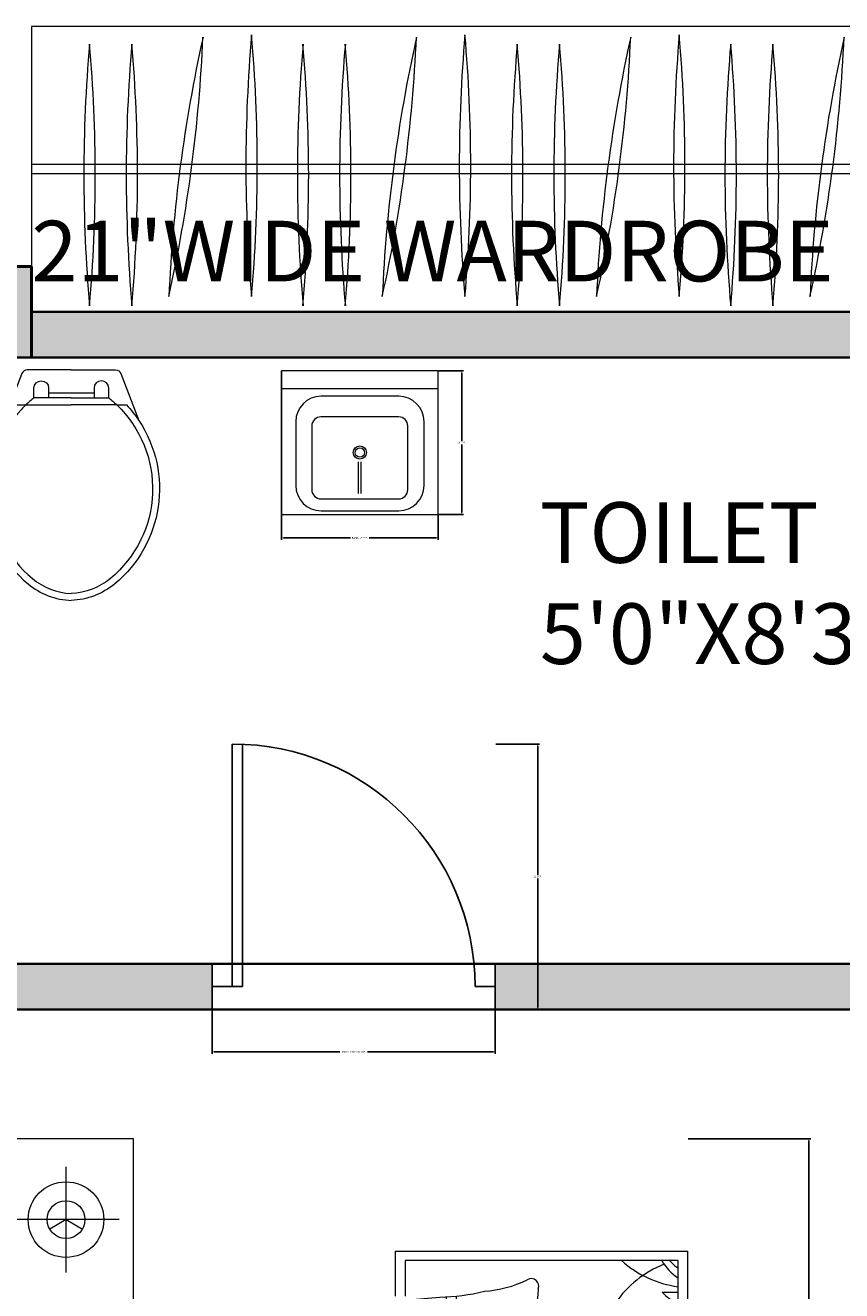
# Model space of a CAD drawing. Units: inches. Extents: x -28 to 485, y -861 to 54.
# Tile 8 of 14: x 36 to 116, y -240 to -115. Entities that reach past the tile are written whole.
import ezdxf

# ---------------------------------------------------------------- set-up
doc = ezdxf.new("R2010")
doc.units = ezdxf.units.IN
doc.header["$MEASUREMENT"] = 0
for name, color, linetype, lineweight in [('A-ANNO-DIMS', 2, 'Continuous', 18), ('A-ANNO-TEXT', 7, 'Continuous', 18), ('A-AREA-IDEN', 7, 'Continuous', 18), ('A-COLS', 7, 'Continuous', 50), ('A-COLS-PATT', 8, 'Continuous', 13), ('A-DOOR', 3, 'Continuous', 25), ('A-FLOR-CASE', 8, 'Continuous', 18), ('A-FLOR-FIXT', 9, 'Continuous', 18), ('A-FURN', 8, 'Continuous', 13), ('A-WALL', 7, 'Continuous', 35), ('A-WALL-PATT', 34, 'Continuous', 13)]:
    doc.layers.add(name, color=color, linetype=linetype, lineweight=lineweight)
doc.styles.get("Standard").update_dxf_attribs({"font": 'arial.ttf'})
doc.dimstyles.get("Standard").update_dxf_attribs({"dimtxt": 0.18, "dimasz": 0.18, "dimexe": 0.18, "dimexo": 0.0625, "dimgap": 0.09, "dimtad": 0, "dimtih": 1, "dimtoh": 1, "dimdec": 0, "dimzin": 0, "dimdsep": 46, "dimlunit": 3, "dimtxsty": 'Standard', "dimcen": 0.09, "dimadec": 0, "dimazin": 0, "dimtfac": 1, "dimtdec": 0, "dimtofl": 0, "dimtmove": 0, "dimatfit": 3, "dimfxl": 1, "dimtolj": 1, "dimtzin": 0, "dimarcsym": 0})

# ---------------------------------------------------------------- blocks, each defined once
blk = doc.blocks.new('М14 600х655')
for p, q in [((-655, 600), (-655, 0)), ((-655, 600), (-655, 0)), ((-655, 0), (-655, 600)), ((0, 600), (-655, 600)), ((0, 0), (0, 600)), ((0, 525), (-655, 525)), ((-165.1, 494.1), (-489.9, 494.1)), ((-595.8, 388.1), (-595.8, 121.3)), ((-165.4, 408.4), (-490.2, 408.4)), ((-59.2, 121.3), (-59.2, 388.1)), ((-528.4, 370.1), (-528.4, 103.3)), ((-127.2, 103.3), (-127.2, 370.1)), ((-333.5, 87.1), (-333.5, 219.6)), ((-321.5, 87.1), (-321.5, 219.6)), ((-490.2, 65.1), (-165.4, 65.1)), ((-655, 0), (-655, 0)), ((-655, 0), (-655, 0)), ((-655, 0), (0, 0)), ((-655, 0), (0, 0)), ((-489.9, 15.4), (-165.1, 15.4))]:
    blk.add_line(p, q)
for radius in [27.6, 19.3]:
    blk.add_circle((-327.5, 258.9), radius)
for centre, radius, start, end in [((-489.9, 388.1), 105.9, 90, 180), ((-165.1, 388.1), 105.9, 0, 90), ((-490.2, 370.1), 38.2, 90, 180), ((-165.4, 370.1), 38.2, 0, 90), ((-489.9, 121.3), 105.9, 180, 270), ((-165.1, 121.3), 105.9, 270, 0), ((-490.2, 103.3), 38.2, 180, 270), ((-165.4, 103.3), 38.2, 270, 0)]:
    blk.add_arc(centre, radius, start, end)
blk = doc.blocks.new('BED-DOUBLE-WITH-NIGHTSTANDS')
for p, q in [((0, 0), (0, 80.08)), ((6.67, 66.84), (6.67, 77.31)), ((11.91, 72.08), (1.44, 72.08)), ((39.26, 64.51), (39.26, 68.96)), ((39.26, 68.96), (68.11, 68.96)), ((68.11, 68.96), (68.11, 10.57)), ((40.19, 68.03), (40.19, 64.5)), ((67.18, 68.03), (40.19, 68.03)), ((67.18, 11.5), (67.18, 68.03)), ((1.03, 64.07), (1.03, 16.02)), ((12.66, 16.02), (12.66, 64.07)), ((15.98, 63.85), (16.38, 35.34)), ((44.25, 64.43), (44.25, 15.09)), ((45.25, 64.51), (45.25, 15.09)), ((16.8, 63.82), (17.22, 34.74)), ((19.33, 63.78), (19.45, 33.37)), ((20.15, 63.78), (20.27, 33.06)), ((59.06, 60.14), (58.15, 60.31)), ((53.12, 56.3), (53.12, 23.78)), ((59.06, 54.54), (58.15, 54.36)), ((12.66, 38.02), (18.76, 33.63)), ((15.04, 27.14), (12.66, 35.87)), ((18.76, 33.63), (23.47, 31.84)), ((23.47, 31.84), (25.57, 31.52)), ((25.57, 31.52), (24.92, 28.93)), ((24.92, 28.93), (23.95, 26.82)), ((17.14, 21.3), (15.04, 27.14)), ((23.95, 26.82), (23.47, 23.25)), ((59.06, 24.99), (58.15, 25.16)), ((23.47, 23.25), (23.14, 19.19)), ((19.41, 18.22), (17.14, 21.3)), ((23.14, 19.19), (23.47, 15.95)), ((59.06, 19.39), (58.15, 19.21)), ((22.82, 15.3), (19.41, 18.22)), ((0, 16.02), (21.98, 16.02)), ((23.47, 15.95), (22.82, 15.3)), ((39.26, 10.57), (39.26, 15.1)), ((40.19, 15.1), (40.19, 11.5)), ((6.67, 13.24), (6.67, 2.78)), ((40.19, 11.5), (67.18, 11.5)), ((68.11, 10.57), (39.26, 10.57)), ((11.91, 8.01), (1.44, 8.01))]:
    blk.add_line(p, q)
for points in [[(0, 64.07), (13.35, 64.07), (13.35, 80.08), (0, 80.08)], [(6.67, 72.08), (5.06, 71.14)], [(6.67, 72.08), (8.29, 71.14)], [(13.35, 16.02), (13.35, 0), (0, 0)], [(6.67, 8.01), (5.06, 8.94)], [(6.67, 8.01), (8.29, 8.94)]]:
    blk.add_lwpolyline(points)
for points in [[(43.62, 64.41, 0.056112), (48.03, 64.99, 0.095341), (52.27, 66.12)], [(2, 59.47, -0.074897), (7.23, 59.37, 0.472817)], [(7.52, 43.09, -0.14099), (2.18, 42.93, -0.235245)], [(7.52, 39.67, 0.14099), (2.18, 39.83, 0.235245)], [(2, 20.62, 0.074897), (7.23, 20.71, -0.472817)], [(30.15, 15.13, 0.001242), (45.35, 15.09, -0.127202), (52.92, 13.49)]]:
    blk.add_lwpolyline(points, format="xyb")
for centre, radius in [((6.67, 72.08), 3.74), ((6.67, 72.08), 1.87), ((64.11, 56.84), 0.204), ((61.96, 55.51), 0.204), ((61.96, 24.02), 0.204), ((64.11, 22.68), 0.204), ((6.67, 8.01), 3.74), ((6.67, 8.01), 1.87)]:
    blk.add_circle(centre, radius)
for centre, radius, start, end in [((69.62, 57.92), 10.46, 111.4092, 145.6135), ((68.59, 75.81), 10.46, 228.1144, 262.255), ((69.99, 70.57), 5.1, 209.8884, 236.5383), ((70.94, 72.4), 6.35, 223.5186, 233.6964), ((52.68, 65.51), 0.73, 336.5219, 123.8264), ((131.01, 58.75), 77.93, 175.2402, 181.8035), ((22.44, 207.63), 143.9, 266.1, 270.9282), ((27.68, 251.44), 187.71, 269.1145, 274.8735), ((60.79, 62.99), 0.867, 76.272, 177.0484), ((61.24, 62.69), 1.16, 20.9613, 102.2885), ((68.81, 67.71), 4.25, 221.0454, 247.4453), ((66.52, 79.36), 14.47, 266.3481, 272.5919), ((58.76, 65.61), 6.06, 203.6453, 236.3329), ((55.85, 62.08), 1.35, 88.9462, 185.5144), ((56.04, 61.53), 1.91, 7.1143, 95.0551), ((59.12, 61.97), 1.2, 19.1312, 189.736), ((60.43, 62.21), 0.737, 126.7319, 206.0245), ((59.47, 64.76), 1.79, 284.7031, 328.6173), ((61.96, 62.49), 1.65, 125.7657, 194.5347), ((53.85, 65.41), 7.32, 332.8176, 347.4827), ((61.86, 63.85), 0.873, 181.7131, 301.5367), ((59, 62.09), 2.64, 2.0648, 41.1598), ((60.59, 63.07), 0.856, 316.2238, 62.3173), ((61.09, 62.57), 0.0682, 20.2667, 316.2271), ((56.85, 62.5), 2.41, 193.079, 274.7067), ((55.32, 60.77), 1.86, 338.5779, 68.4181), ((55.62, 61.86), 2.33, 305.9599, 357.6409), ((56.48, 64.35), 3.78, 288.2955, 328.7386), ((58.76, 62.26), 1.5, 285.6955, 4.031), ((60.76, 60.64), 1.6, 128.4175, 173.8338), ((61.51, 62.18), 0.13, 168.5166, 2.0648), ((61.45, 62.19), 0.0631, 52.0591, 168.5166), ((53.71, 63.39), 3.32, 259.249, 301.1782), ((55.15, 57.49), 3.09, 85.2696, 124.215), ((57.33, 61.13), 1.99, 196.8663, 330.0915), ((55.15, 57.49), 3.09, 53.6555, 57.2989), ((56.78, 64.39), 4.3, 273.4924, 303.7117), ((-760.15, 15.33), 763.42, 2.85022, 3.31479), ((9.33, 49.26), 10.32, 78.2417, 114.8684), ((1.06, 56.61), 10.73, 348.9631, 14.8961), ((54, 59.28), 0.964, 127.675, 162.5814), ((54, 59.28), 0.964, 196.6343, 225.5483), ((54.57, 60.82), 2.55, 240.8249, 340.7178), ((53.81, 59.69), 1.2, 246.1646, 318.4347), ((55.03, 61.2), 2.3, 240.0851, 262.564), ((55.94, 57.8), 1.64, 74.8529, 138.4347), ((56.5, 59.87), 0.497, 254.8529, 12.6959), ((60.19, 59.12), 0.158, 125.0752, 284.7644), ((60.43, 59.18), 0.34, 127.3642, 168.4363), ((60.17, 59.45), 0.49, 277.4968, 341.2737), ((60.56, 59.22), 0.195, 88.1325, 178.8919), ((60.95, 59.02), 0.422, 136.3462, 189.6513), ((60.71, 58.98), 0.176, 189.6513, 312.3208), ((60.75, 59.46), 0.204, 183.2768, 356.7232), ((61.39, 59.1), 0.668, 164.2829, 186.9148), ((60.6, 59.09), 0.334, 312.3208, 40.2111), ((61.31, 59.47), 0.474, 201.6382, 274.947), ((60.68, 58.82), 0.619, 42.3896, 66.5724), ((66.93, 63.72), 7.6, 217.9541, 226.8459), ((61.13, 59.18), 0.337, 10.9597, 52.2379), ((61.33, 59.15), 0.156, 274.947, 37.5263), ((62.33, 58.47), 0.42, 115.5379, 168.6744), ((60.9, 59.07), 1.27, 329.344, 349.7412), ((59.89, 58.78), 2.26, 352.8698, 1.6736), ((61.28, 51.56), 6.63, 110.1059, 116.9968), ((59.01, 57.53), 0.163, 83.9457, 185.6216), ((58.36, 57.69), 0.671, 328.836, 0.8141), ((58.71, 57.49), 0.384, 306.5232, 32.4668), ((59.16, 57.79), 0.163, 112.5583, 214.2343), ((59.06, 58.08), 0.384, 265.7131, 351.6568), ((58.72, 58.29), 0.671, 297.3659, 329.344), ((58.21, 58.87), 1.29, 313.6929, 321.7899), ((59.64, 57.99), 0.42, 115.5379, 168.6744), ((58.21, 58.6), 1.27, 329.344, 349.7412), ((61.28, 51.56), 6.63, 86.1723, 106.4158), ((57.2, 58.31), 2.26, 352.8698, 1.6736), ((61.86, 58.27), 0.163, 112.5583, 214.2343), ((61.75, 58.56), 0.384, 265.7131, 351.6568), ((61.42, 58.77), 0.671, 297.3659, 329.344), ((61.45, 54.86), 3.33, 60.7959, 85.244), ((54.37, 50.07), 10.94, 37.8256, 47.7588), ((60.91, 59.35), 1.29, 313.6929, 321.7899), ((63.07, 58.33), 0.228, 33.0979, 123.1364), ((58.05, 55.12), 5.96, 31.1156, 34.8118), ((62.74, 57.94), 0.617, 2.3172, 70.5201), ((62.44, 57.27), 0.93, 310.9365, 22.7695), ((63.25, 57.78), 0.178, 135.7354, 318.1297), ((62.95, 58.07), 0.236, 315.7354, 31.1156), ((62.75, 57.57), 0.547, 319.3812, 5.5456), ((63.38, 57.79), 0.178, 68.2452, 250.6395), ((62.97, 58), 0.531, 352.6008, 57.1845), ((64.87, 54.44), 3.55, 111.7087, 116.2181), ((61.45, 54.86), 3.33, 47.5083, 55.9967), ((63.48, 58.12), 0.531, 252.8042, 349.6943), ((62.97, 57.17), 0.565, 331.1838, 51.6792), ((63.53, 58.17), 0.236, 248.2452, 323.6254), ((63.33, 58.31), 0.617, 291.7087, 3.0299), ((58.93, 61.56), 5.96, 323.6254, 327.3216), ((63.81, 58.16), 0.228, 325.6077, 55.6462), ((54.57, 53.85), 2.55, 19.2822, 119.1751), ((57.16, 57.12), 0.251, 169.5864, 349.5616), ((57.25, 57.11), 0.154, 349.5616, 167.2949), ((59.06, 57.02), 0.42, 129.5056, 182.6421), ((57.85, 58), 1.27, 308.4388, 328.836), ((57.63, 59.02), 2.26, 296.5064, 305.3102), ((57.61, 57.86), 1.29, 336.3901, 344.4871), ((61.66, 57.07), 0.93, 253.6301, 325.4631), ((61.92, 55.78), 0.658, 82.0748, 142.6895), ((61.87, 56.57), 0.565, 273.8774, 357.1501), ((62.09, 56.97), 0.547, 262.0748, 308.2393), ((62.97, 56.41), 0.565, 181.4625, 249.4747), ((62.87, 56.86), 0.547, 215.1128, 261.2773), ((63.31, 56.83), 0.93, 197.889, 269.722), ((65.87, 54.52), 3.99, 130.182, 149.456), ((63.67, 56.79), 0.658, 139.3812, 199.9959), ((62.87, 57.22), 0.675, 285.6484, 332.2957), ((63.55, 56.5), 0.158, 125.0752, 284.7644), ((63.8, 56.56), 0.34, 93.635, 168.4363), ((63.75, 57.1), 0.2, 138.2946, 276.2474), ((63.53, 56.83), 0.49, 277.4968, 341.2737), ((63.83, 57.07), 0.278, 358.5719, 143.8954), ((63.92, 56.61), 0.195, 88.1325, 178.8919), ((63.99, 57.29), 0.281, 208.8493, 269.9355), ((63.75, 57.22), 0.321, 274.2123, 318.1587), ((64.31, 56.4), 0.422, 136.3462, 189.6513), ((64.75, 56.48), 0.668, 164.2829, 186.9148), ((64.73, 56.9), 0.643, 121.9501, 165.2442), ((63.96, 56.47), 0.334, 312.3208, 40.2111), ((64.67, 56.85), 0.474, 201.6382, 274.947), ((64.28, 57.14), 0.135, 262.868, 7.094), ((64.04, 56.2), 0.619, 42.3896, 66.5724), ((64.27, 57.26), 0.403, 278.5614, 22.5914), ((64.49, 56.56), 0.337, 10.9597, 118.7804), ((64.49, 57.27), 0.202, 44.3732, 121.9501), ((64.7, 56.53), 0.156, 274.947, 37.5263), ((54, 55.39), 0.964, 134.4517, 156.7144), ((53.81, 54.99), 1.2, 41.5653, 113.8354), ((55.03, 53.47), 2.3, 97.436, 119.9149), ((55.94, 56.87), 1.64, 221.5653, 285.1471), ((57.33, 53.55), 1.99, 29.9085, 163.1337), ((56.5, 54.81), 0.497, 347.3041, 105.1471), ((61.4, 55.17), 0.158, 125.0752, 284.7644), ((61.65, 55.23), 0.34, 93.635, 168.4363), ((61.85, 56.68), 0.675, 228.342, 274.9894), ((61.6, 55.76), 0.2, 138.2946, 276.2474), ((61.38, 55.5), 0.49, 277.4968, 341.2737), ((61.68, 55.73), 0.278, 358.5719, 143.8954), ((61.77, 55.27), 0.195, 88.1325, 178.8919), ((61.84, 55.95), 0.281, 208.8493, 269.9355), ((61.6, 55.89), 0.321, 274.2123, 318.1587), ((62.16, 55.06), 0.422, 136.3462, 189.6513), ((62.6, 55.14), 0.668, 164.2829, 186.9148), ((62.58, 55.56), 0.643, 121.9501, 165.2442), ((61.81, 55.14), 0.334, 312.3208, 40.2111), ((62.52, 55.52), 0.474, 201.6382, 274.947), ((62.13, 55.81), 0.135, 262.868, 7.094), ((61.89, 54.87), 0.619, 42.3896, 66.5724), ((62.12, 55.92), 0.403, 278.5614, 22.5914), ((62.34, 55.23), 0.337, 10.9597, 118.7804), ((65.87, 54.52), 3.99, 156.1523, 156.9499), ((62.34, 55.94), 0.202, 44.3732, 121.9501), ((62.55, 55.2), 0.156, 274.947, 37.5263), ((63.02, 56.51), 0.675, 248.3627, 295.0101), ((62.69, 55.67), 0.658, 20.6625, 81.2773), ((64.07, 56.36), 0.176, 189.6513, 312.3208), ((1.85, 51.98), 10.19, 333.8761, 16.1746), ((54, 55.39), 0.964, 203.2856, 232.325), ((53.71, 51.28), 3.32, 58.8218, 100.2867), ((58.76, 49.06), 6.06, 123.6671, 158.5059), ((55.15, 57.18), 3.09, 235.785, 274.7304), ((56.85, 52.18), 2.41, 85.2933, 166.921), ((55.32, 53.9), 1.86, 291.5819, 21.4221), ((55.15, 57.18), 3.09, 302.7011, 306.3445), ((55.62, 52.81), 2.33, 2.3591, 54.0401), ((56.78, 50.29), 4.3, 56.2883, 86.5076), ((56.48, 50.32), 3.78, 31.2614, 71.7045), ((60.76, 54.03), 1.6, 186.1662, 231.5825), ((58.76, 52.42), 1.5, 355.969, 74.3045), ((61.92, 55.02), 0.176, 189.6513, 312.3208), ((65.87, 54.52), 3.99, 175.2415, 182.8929), ((16.01, 49.96), 14.08, 166.3427, 191.1841), ((55.85, 52.59), 1.35, 174.4856, 271.0538), ((56.04, 53.15), 1.91, 264.9449, 352.8857), ((59.12, 52.71), 1.2, 170.264, 340.8688), ((60.43, 52.46), 0.737, 153.9755, 233.2681), ((61.96, 52.19), 1.65, 165.4653, 234.2343), ((53.85, 49.26), 7.32, 12.5173, 27.1824), ((61.51, 52.5), 0.13, 357.9352, 191.4834), ((60.79, 51.69), 0.867, 182.9516, 283.728), ((59.47, 49.92), 1.79, 31.3827, 75.2969), ((59, 52.59), 2.64, 318.8402, 357.9352), ((60.59, 51.6), 0.856, 297.6827, 43.7762), ((61.86, 50.82), 0.873, 58.4633, 178.2869), ((61.24, 51.98), 1.16, 257.7115, 339.0387), ((61.13, 52.12), 0.113, 43.7762, 339.7183), ((61.45, 52.48), 0.0631, 191.4834, 307.9409), ((69.62, 56.75), 10.46, 214.3865, 248.5908), ((68.81, 46.96), 4.25, 112.5547, 138.9546), ((66.17, 41.19), 8.09, 82.8636, 171.8197), ((66.52, 35.31), 14.47, 87.4081, 93.6519), ((66.74, 46.53), 1.88, 76.3898, 169.0739), ((74.19, 42.33), 10.46, 152.5854, 175.5377), ((66.48, 45.12), 2.37, 72.8609, 131.9049), ((65.43, 42.24), 4.68, 68.117, 96.6195), ((72.68, 45.26), 5.75, 162.9798, 196.4569), ((5.99, 44.03), 3.96, 153.3437, 196.1026), ((7.37, 44.56), 4.25, 335.0183, 18.5407), ((75.64, 42.98), 8.5, 174.3643, 175.6213), ((10.2, 52.53), 9.81, 254.1707, 275.9871), ((58.94, 41.49), 1.16, 50.8855, 132.2127), ((64.01, 42.31), 0.867, 106.1963, 206.9726), ((61.98, 43.19), 1.79, 314.6273, 358.5415), ((65.27, 42.46), 1.65, 155.6899, 224.4589), ((64.54, 42.29), 1.16, 50.8855, 132.2127), ((64.51, 43.6), 0.873, 211.6373, 331.4609), ((63.8, 42.29), 0.856, 346.148, 92.2415), ((62.91, 40.64), 2.64, 31.989, 71.0841), ((56.78, 40.96), 7.32, 2.7418, 17.407), ((81.47, 38.5), 15.2, 160.0972, 160.2783), ((58.4, 41.51), 0.867, 106.1963, 206.9726), ((56.38, 42.39), 1.79, 314.6273, 358.5415), ((59.67, 41.66), 1.65, 155.6899, 224.4589), ((59.67, 40.53), 1.65, 135.5411, 204.3101), ((58.91, 42.8), 0.873, 211.6373, 331.4609), ((58.2, 41.49), 0.856, 346.148, 92.2415), ((57.3, 39.84), 2.64, 31.989, 71.0841), ((51.18, 40.16), 7.32, 2.7418, 17.407), ((51.18, 42.04), 7.32, 342.593, 357.2582), ((58.87, 41.3), 0.0682, 50.1909, 346.0209), ((64.47, 42.1), 0.0682, 50.1909, 346.0209), ((64.98, 41.95), 0.0631, 81.9833, 198.4408), ((65.04, 41.98), 0.13, 198.4408, 31.989), ((58.4, 40.68), 0.867, 153.0274, 253.8037), ((56.38, 39.81), 1.79, 1.4585, 45.3727), ((57.3, 42.35), 2.64, 288.9159, 328.011), ((58.2, 40.71), 0.856, 267.7585, 13.852), ((58.91, 39.39), 0.873, 28.5391, 148.3627), ((58.92, 40.88), 0.113, 13.852, 309.9245), ((59.44, 41.17), 0.13, 198.4408, 31.989), ((59.37, 41.15), 0.0631, 81.9833, 198.4408), ((59.44, 41.02), 0.13, 328.011, 161.5592), ((59.37, 41.04), 0.0631, 161.5592, 278.0167), ((64.01, 39.88), 0.867, 153.0274, 253.8037), ((61.98, 39.01), 1.79, 1.4585, 45.3727), ((65.27, 39.73), 1.65, 135.5411, 204.3101), ((56.78, 41.24), 7.32, 342.593, 357.2582), ((62.91, 41.55), 2.64, 288.9159, 328.011), ((63.8, 39.91), 0.856, 267.7585, 13.852), ((64.52, 40.08), 0.113, 13.852, 309.9245), ((64.98, 40.24), 0.0631, 161.5592, 278.0167), ((65.04, 40.22), 0.13, 328.011, 161.5592), ((16.3, 37.72), 14.27, 171.5249, 193.96), ((10.2, 30.23), 9.81, 84.0129, 105.8293), ((-2.51, 36.66), 14.12, 349.8617, 13.6238), ((58.94, 40.71), 1.16, 227.7873, 309.1145), ((68.59, 40.66), 10.46, 184.4623, 262.255), ((64.51, 38.59), 0.873, 28.5391, 148.3627), ((64.54, 39.91), 1.16, 227.7873, 309.1145), ((74.19, 39.86), 10.46, 184.4623, 207.4146), ((72.68, 36.94), 5.75, 163.5431, 197.0202), ((75.64, 39.22), 8.5, 184.3787, 185.6357), ((81.47, 43.7), 15.2, 199.7217, 199.9028), ((30.98, 31.59), 29.04, 172.2196, 189.497), ((-6.57, 29.12), 18.61, 348.0397, 19.2615), ((69.99, 35.42), 5.1, 181.272, 236.5383), ((72.72, 40.59), 9.45, 214.0123, 234.053), ((70.94, 37.25), 6.35, 197.8504, 233.6964), ((-4.69, 37.08), 31.06, 340.1194, 349.3383), ((25.64, 31.34), 0.193, 358.8623, 109.7536), ((69.62, 22.77), 10.46, 111.4092, 145.6135), ((66.52, 44.21), 14.47, 266.3481, 272.5919), ((68.81, 32.56), 4.25, 221.0454, 247.4453), ((58.76, 30.46), 6.06, 201.4941, 236.3329), ((55.85, 26.93), 1.35, 88.9462, 185.5144), ((56.04, 26.38), 1.91, 7.1143, 95.0551), ((59.12, 26.82), 1.2, 19.1312, 189.736), ((60.43, 27.07), 0.737, 126.7319, 206.0245), ((60.79, 27.84), 0.867, 76.272, 177.0484), ((59.47, 29.61), 1.79, 284.7031, 328.6173), ((61.96, 27.34), 1.65, 125.7657, 194.5347), ((53.85, 30.27), 7.32, 332.8176, 347.4827), ((61.24, 27.55), 1.16, 20.9613, 102.2885), ((60.59, 27.92), 0.856, 316.2238, 62.3173), ((59, 26.94), 2.64, 2.0648, 41.1598), ((61.86, 28.71), 0.873, 181.7131, 301.5367), ((-760.15, 64.76), 763.42, 356.68521, 357.14978), ((30.48, 23.89), 6.52, 156.2616, 191.3392), ((56.85, 27.35), 2.41, 193.079, 274.7067), ((55.32, 25.63), 1.86, 338.5779, 68.4181), ((55.62, 26.71), 2.33, 305.9599, 357.6409), ((56.48, 29.2), 3.78, 288.2955, 328.7386), ((58.76, 27.11), 1.5, 285.6955, 4.031), ((60.76, 25.49), 1.6, 128.4175, 173.8338), ((61.09, 27.42), 0.0682, 20.2667, 316.2271), ((61.51, 27.03), 0.13, 168.5166, 2.0648), ((61.45, 27.04), 0.0631, 52.0591, 168.5166), ((1.06, 23.47), 10.73, 345.1039, 11.0369), ((53.71, 28.24), 3.32, 259.7133, 301.1782), ((55.15, 22.34), 3.09, 85.2696, 124.215), ((57.33, 25.98), 1.99, 196.8663, 330.0915), ((56.78, 29.24), 4.3, 273.4924, 303.7117), ((65.87, 25.01), 3.99, 177.1071, 184.7585), ((136.48, 22.83), 83.37, 179.3433, 185.6887), ((54, 24.13), 0.964, 127.675, 156.7144), ((54.57, 25.67), 2.55, 240.8249, 340.7178), ((55.03, 26.06), 2.3, 240.0851, 262.564), ((55.94, 22.65), 1.64, 74.8529, 138.4347), ((56.5, 24.72), 0.497, 254.8529, 12.6959), ((55.15, 22.34), 3.09, 53.6555, 57.2989), ((61.4, 24.36), 0.158, 75.2356, 234.9248), ((61.65, 24.3), 0.34, 191.5637, 266.365), ((61.6, 23.76), 0.2, 83.7526, 221.7054), ((61.38, 24.03), 0.49, 18.7263, 82.5032), ((61.68, 23.79), 0.278, 216.1046, 1.4281), ((61.77, 24.25), 0.195, 181.1081, 271.8675), ((61.84, 23.57), 0.281, 90.0645, 151.1507), ((61.6, 23.64), 0.321, 41.8413, 85.7877), ((61.92, 24.5), 0.176, 47.6792, 170.3487), ((62.16, 24.46), 0.422, 170.3487, 223.6538), ((62.6, 24.38), 0.668, 173.0852, 195.7171), ((62.58, 23.96), 0.643, 194.7558, 238.0499), ((61.81, 24.39), 0.334, 319.7889, 47.6792), ((62.52, 24.01), 0.474, 85.053, 158.3618), ((62.13, 23.71), 0.135, 352.906, 97.132), ((61.89, 24.66), 0.619, 293.4276, 317.6104), ((62.34, 24.29), 0.337, 241.2196, 349.0403), ((62.12, 23.6), 0.403, 337.4086, 81.4386), ((62.55, 24.33), 0.156, 322.4737, 85.053), ((-5.54, 16.67), 30.23, 357.4519, 11.3392), ((54, 24.13), 0.964, 203.229, 225.5483), ((53.81, 24.54), 1.2, 246.1646, 318.4347), ((57.16, 22.4), 0.251, 10.4384, 190.4136), ((61.85, 22.84), 0.675, 85.0106, 131.658), ((61.66, 22.46), 0.93, 34.5369, 106.3699), ((61.92, 23.75), 0.658, 217.3105, 277.9252), ((54.37, 29.45), 10.94, 312.2412, 322.1744), ((61.87, 22.95), 0.565, 2.8499, 86.1226), ((62.09, 22.55), 0.547, 51.7607, 97.9252), ((65.87, 25.01), 3.99, 203.0501, 203.8477), ((62.34, 23.59), 0.202, 238.0499, 315.6268), ((62.97, 23.11), 0.565, 110.5253, 178.5375), ((63.31, 22.7), 0.93, 90.278, 162.111), ((62.87, 22.67), 0.547, 98.7227, 144.8872), ((65.87, 25.01), 3.99, 210.544, 229.818), ((63.02, 23.01), 0.675, 64.9899, 111.6373), ((62.69, 23.86), 0.658, 278.7227, 339.3375), ((63.67, 22.74), 0.658, 160.0041, 220.6188), ((62.44, 22.26), 0.93, 337.2305, 49.0635), ((62.87, 22.31), 0.675, 27.7043, 74.3516), ((62.97, 22.35), 0.565, 308.3208, 28.8162), ((63.55, 23.03), 0.158, 75.2356, 234.9248), ((63.8, 22.96), 0.34, 191.5637, 266.365), ((63.75, 22.43), 0.2, 83.7526, 221.7054), ((63.53, 22.69), 0.49, 18.7263, 82.5032), ((63.92, 22.92), 0.195, 181.1081, 271.8675), ((63.75, 22.31), 0.321, 41.8413, 85.7877), ((64.07, 23.17), 0.176, 47.6792, 170.3487), ((64.31, 23.13), 0.422, 170.3487, 223.6538), ((64.75, 23.05), 0.668, 173.0852, 195.7171), ((63.96, 23.05), 0.334, 319.7889, 47.6792), ((64.67, 22.68), 0.474, 85.053, 158.3618), ((64.04, 23.32), 0.619, 293.4276, 317.6104), ((64.49, 22.96), 0.337, 241.2196, 349.0403), ((64.27, 22.27), 0.403, 337.4086, 81.4386), ((64.7, 22.99), 0.156, 322.4737, 85.053), ((9.33, 30.82), 10.32, 245.1316, 281.7583), ((57.25, 22.42), 0.154, 192.7051, 10.4384), ((61.28, 27.97), 6.63, 243.0032, 249.8941), ((57.85, 21.53), 1.27, 31.164, 51.5612), ((59.06, 22.5), 0.42, 177.3579, 230.4944), ((57.63, 20.5), 2.26, 54.6898, 63.4936), ((57.61, 21.66), 1.29, 15.5129, 23.6099), ((59.01, 21.99), 0.163, 174.3784, 276.0543), ((58.71, 22.03), 0.384, 327.5332, 53.4768), ((58.36, 21.84), 0.671, 359.1859, 31.164), ((59.16, 21.74), 0.163, 145.7657, 247.4417), ((59.06, 21.45), 0.384, 8.3432, 94.2869), ((58.72, 21.23), 0.671, 30.656, 62.6341), ((58.21, 20.66), 1.29, 38.2101, 46.3071), ((59.64, 21.53), 0.42, 191.3256, 244.4621), ((58.21, 20.93), 1.27, 10.2588, 30.656), ((61.28, 27.97), 6.63, 253.5842, 273.8277), ((57.2, 21.22), 2.26, 358.3264, 7.1302), ((66.93, 15.8), 7.6, 133.1541, 142.0459), ((61.86, 21.26), 0.163, 145.7657, 247.4417), ((61.45, 24.67), 3.33, 274.756, 299.2041), ((61.75, 20.97), 0.384, 8.3432, 94.2869), ((61.42, 20.76), 0.671, 30.656, 62.6341), ((62.74, 21.59), 0.617, 289.4799, 357.6828), ((58.05, 24.41), 5.96, 325.1882, 328.8844), ((63.25, 21.74), 0.178, 41.8703, 224.2646), ((62.95, 21.45), 0.236, 328.8844, 44.2646), ((62.75, 21.95), 0.547, 354.4544, 40.6188), ((63.38, 21.74), 0.178, 109.3605, 291.7548), ((62.97, 21.52), 0.531, 302.8155, 7.3992), ((64.87, 25.09), 3.55, 243.7819, 248.2913), ((61.45, 24.67), 3.33, 304.0033, 312.4917), ((63.48, 21.4), 0.531, 10.3057, 107.1958), ((63.53, 21.36), 0.236, 36.3746, 111.7548), ((63.33, 21.21), 0.617, 356.9701, 68.2913), ((63.83, 22.46), 0.278, 216.1046, 1.4281), ((58.93, 17.96), 5.96, 32.6784, 36.3746), ((63.99, 22.24), 0.281, 90.0645, 151.1507), ((63.81, 21.37), 0.228, 304.3538, 34.3923), ((64.73, 22.63), 0.643, 194.7558, 238.0499), ((64.28, 22.38), 0.135, 352.906, 97.132), ((64.49, 22.25), 0.202, 238.0499, 315.6268), ((54, 20.25), 0.964, 134.4517, 153.558), ((54.57, 18.71), 2.55, 19.2822, 119.1751), ((53.81, 19.84), 1.2, 41.5653, 113.8354), ((55.03, 18.32), 2.3, 97.436, 119.9149), ((55.94, 21.72), 1.64, 221.5653, 285.1471), ((57.33, 18.4), 1.99, 29.9085, 163.1337), ((56.5, 19.66), 0.497, 347.3041, 105.1471), ((60.19, 20.41), 0.158, 75.2356, 234.9248), ((60.43, 20.35), 0.34, 191.5637, 232.6358), ((60.17, 20.07), 0.49, 18.7263, 82.5032), ((60.56, 20.3), 0.195, 181.1081, 271.8675), ((60.71, 20.55), 0.176, 47.6792, 170.3487), ((60.95, 20.51), 0.422, 170.3487, 223.6538), ((60.75, 20.06), 0.204, 3.2768, 176.7232), ((61.39, 20.43), 0.668, 173.0852, 195.7171), ((60.6, 20.43), 0.334, 319.7889, 47.6792), ((61.31, 20.06), 0.474, 85.053, 158.3618), ((60.68, 20.7), 0.619, 293.4276, 317.6104), ((61.13, 20.34), 0.337, 307.7621, 349.0403), ((61.33, 20.37), 0.156, 322.4737, 85.053), ((60.91, 20.18), 1.29, 38.2101, 46.3071), ((62.33, 21.06), 0.42, 191.3256, 244.4621), ((60.9, 20.45), 1.27, 10.2588, 30.656), ((59.89, 20.74), 2.26, 358.3264, 7.1302), ((63.07, 21.2), 0.228, 236.8636, 326.9021), ((54, 20.25), 0.964, 210.0293, 232.325), ((53.71, 16.14), 3.32, 58.8218, 99.1554), ((58.76, 13.91), 6.06, 123.6671, 153.2997), ((55.15, 22.04), 3.09, 235.785, 274.7304), ((56.85, 17.03), 2.41, 85.2933, 166.921), ((55.32, 18.75), 1.86, 291.5819, 21.4221), ((55.15, 22.04), 3.09, 302.7011, 306.3445), ((55.62, 17.67), 2.33, 2.3591, 54.0401), ((56.78, 15.14), 4.3, 56.2883, 86.5076), ((55.85, 17.44), 1.35, 174.4856, 271.0538), ((56.04, 18), 1.91, 264.9449, 352.8857), ((56.48, 15.18), 3.78, 31.2614, 71.7045), ((59.12, 17.56), 1.2, 170.264, 340.8688), ((58.76, 17.27), 1.5, 355.969, 74.3045), ((60.76, 18.89), 1.6, 186.1662, 231.5825), ((60.43, 17.31), 0.737, 153.9755, 233.2681), ((59.47, 14.77), 1.79, 31.3827, 75.2969), ((60.79, 16.54), 0.867, 182.9516, 283.728), ((61.96, 17.04), 1.65, 165.4653, 234.2343), ((53.85, 14.11), 7.32, 12.5173, 27.1824), ((59, 17.44), 2.64, 318.8402, 357.9352), ((60.59, 16.46), 0.856, 297.6827, 43.7762), ((61.86, 15.67), 0.873, 58.4633, 178.2869), ((61.24, 16.83), 1.16, 257.7115, 339.0387), ((61.13, 16.97), 0.113, 43.7762, 339.7183), ((61.51, 17.35), 0.13, 357.9352, 191.4834), ((61.45, 17.33), 0.0631, 191.4834, 307.9409), ((24.81, -58.13), 73.46, 85.8294, 91.553), ((69.62, 21.6), 10.46, 214.3865, 248.5908), ((68.81, 11.81), 4.25, 112.5547, 138.9546), ((52.87, 14.23), 0.739, 273.98, 27.3412), ((68.59, 3.71), 10.46, 97.745, 131.8856), ((66.52, 0.17), 14.47, 87.4081, 93.6519), ((69.99, 8.96), 5.1, 123.4617, 150.1116), ((70.94, 7.13), 6.35, 126.3036, 136.4814)]:
    blk.add_arc(centre, radius, start, end)
blk = doc.blocks.new('WARDROBE-HANGING')
for p, q in [((84.7, 28.23), (0, 28.23)), ((0, 28.23), (0, 0)), ((84.7, 28.23), (84.7, 0)), ((84.7, 14.59), (0, 14.59)), ((84.7, 13.65), (0, 13.65)), ((84.7, 0), (0, 0))]:
    blk.add_line(p, q)
for centre, start, end in [((153.74, 13.55), 175.0028, 184.9972), ((-142.25, 13.55), 355.0028, 4.9972), ((157.93, 13.55), 175.0028, 184.9972), ((-138.07, 13.55), 355.0028, 4.9972), ((-131.46, 33.65), 347.508, 357.5023), ((162.01, -4.96), 167.508, 177.5023), ((169.76, 14.46), 175.0028, 184.9972), ((-126.23, 14.46), 355.0028, 4.9972), ((174.85, 13.55), 175.0028, 184.9972), ((-121.15, 13.55), 355.0028, 4.9972), ((179.03, 13.55), 175.0028, 184.9972), ((-116.97, 13.55), 355.0028, 4.9972), ((-110.36, 33.65), 347.508, 357.5023), ((183.11, -4.96), 167.508, 177.5023), ((190.86, 14.46), 175.0028, 184.9972), ((-105.13, 14.46), 355.0028, 4.9972), ((196.03, 13.55), 175.0028, 184.9972), ((-99.97, 13.55), 355.0028, 4.9972), ((200.21, 13.55), 175.0028, 184.9972), ((-95.78, 13.55), 355.0028, 4.9972), ((204.29, -4.96), 167.508, 177.5023), ((-89.17, 33.65), 347.508, 357.5023), ((212.05, 14.46), 175.0028, 184.9972), ((-83.95, 14.46), 355.0028, 4.9972), ((217.13, 13.55), 175.0028, 184.9972), ((-78.86, 13.55), 355.0028, 4.9972), ((221.31, 13.55), 175.0028, 184.9972), ((-74.68, 13.55), 355.0028, 4.9972), ((225.4, -4.96), 167.508, 177.5023), ((-68.07, 33.65), 347.508, 357.5023)]:
    blk.add_arc(centre, 148.56, start, end)
blk = doc.blocks.new('WC-FLOOR-MOUNTED')
for p, q in [((3.27, 19.35), (4.23, 19.35)), ((4.23, 19.35), (8.71, 19.35)), ((13.2, 19.35), (8.71, 19.35)), ((13.2, 19.35), (14.16, 19.35))]:
    blk.add_line(p, q)
for points in [[(8.71, 22.81), (4.36, 22.81, 0.31031), (3.82, 22.44), (2.03, 17.79, 0.209071)], [(8.71, 22.81), (13.07, 22.81, -0.31031), (13.6, 22.44), (15.39, 17.79, -0.209071)], [(5.01, 20.04), (5.01, 21, -1), (6.47, 21), (6.47, 20.5)], [(12.41, 20.04), (12.41, 21, 1), (10.96, 21), (10.96, 20.5)], [(5.01, 20.04, 0.022712), (4.23, 19.35, 0.162618)], [(8.71, 20.04), (5.01, 20.04, 0.022712)], [(8.71, 20.04), (12.41, 20.04, -0.476108)], [(12.41, 20.04, -0.022712), (13.2, 19.35, -0.162618)], [(3.77, 18.89, 0.431639), (4.86, 2.17, 0.162618), (8.71, 0.68, 0.470877)], [(3.27, 19.35, 0.040937), (2.03, 17.79, 0.163732)], [(4.23, 19.35, 0.014165), (3.77, 18.89, 0.162618)], [(13.2, 19.35, -0.448546), (12.57, 2.17, -0.162618), (8.71, 0.68, -0.470877)], [(14.16, 19.35, -0.040937), (15.39, 17.79, -0.163732)], [(2.03, 17.79, 0.383919), (4.43, 1.64, 0.163732), (8.71, 0, 0.359733)], [(15.39, 17.79, -0.383919), (13, 1.64, -0.163732), (8.71, 0, -0.359733)]]:
    blk.add_lwpolyline(points, format="xyb")
for points in [[(10.96, 20.5), (6.47, 20.5)], [(6.47, 20.5), (6.47, 20.04)], [(10.96, 20.5), (10.96, 20.04)]]:
    blk.add_lwpolyline(points)
blk = doc.blocks.new('DOOR-SWING-24')
for p, q in [((2, 2.25), (2, 26.25)), ((3, 2.25), (3, 26.25)), ((0, 4.5), (0, 0)), ((28, 2.25), (28, 4.5)), ((0, 2.25), (2, 2.25)), ((2, 2.25), (3, 2.25)), ((26, 2.25), (28, 2.25)), ((28, 2.25), (28, 0))]:
    blk.add_line(p, q)
blk.add_arc((2, 2.25), 24, 0, 90)
blk = doc.blocks.new('*D22')
at = {"layer": 'A-ANNO-DIMS', "color": 0, "lineweight": -2, "transparency": 16777216}
for p, q in [((54.14, -211.93), (54.14, -216.25)), ((82.14, -211.93), (82.14, -216.25)), ((54.32, -216.07), (66.78, -216.07)), ((81.96, -216.07), (69.51, -216.07))]:
    blk.add_line(p, q, dxfattribs=at)
at = {"layer": 'A-ANNO-DIMS', "color": 0, "transparency": 16777216}
for points in [[(54.32, -216.04), (54.32, -216.1), (54.14, -216.07)], [(81.96, -216.04), (81.96, -216.1), (82.14, -216.07)]]:
    blk.add_solid(points, dxfattribs=at)
at = {"layer": 'Defpoints', "color": 0, "transparency": 16777216}
for p in [(54.14, -211.87), (82.14, -211.87), (82.14, -216.07)]:
    blk.add_point(p, dxfattribs=at)
at = {"layer": 'A-ANNO-DIMS', "color": 0, "transparency": 16777216, "insert": (68.14, -216.07), "char_height": 0.18, "attachment_point": 5}
blk.add_mtext('\\A1;ROOM DOOR 28 TYP.', dxfattribs=at)
blk = doc.blocks.new('*D23')
at = {"layer": 'A-ANNO-DIMS', "color": 0, "lineweight": -2, "transparency": 16777216}
for p, q in [((82.21, -185.62), (86.52, -185.62)), ((86.34, -185.8), (86.34, -198.56)), ((86.34, -211.69), (86.34, -198.92)), ((82.21, -211.87), (86.52, -211.87))]:
    blk.add_line(p, q, dxfattribs=at)
at = {"layer": 'A-ANNO-DIMS', "color": 0, "transparency": 16777216}
for points in [[(86.31, -185.8), (86.37, -185.8), (86.34, -185.62)], [(86.31, -211.69), (86.37, -211.69), (86.34, -211.87)]]:
    blk.add_solid(points, dxfattribs=at)
at = {"layer": 'Defpoints', "color": 0, "transparency": 16777216}
for p in [(82.14, -185.62), (86.34, -185.62), (82.14, -211.87)]:
    blk.add_point(p, dxfattribs=at)
at = {"layer": 'A-ANNO-DIMS', "color": 0, "transparency": 16777216, "insert": (86.34, -198.74), "char_height": 0.18, "attachment_point": 5}
blk.add_mtext('\\A1;26 TYP.', dxfattribs=at)
blk = doc.blocks.new('*D24')
at = {"layer": 'A-ANNO-DIMS', "color": 0, "lineweight": -2, "transparency": 16777216}
for p, q in [((101.2, -224.66), (113.33, -224.66)), ((113.15, -224.84), (113.15, -264.52)), ((113.15, -304.56), (113.15, -264.88)), ((101.2, -304.74), (113.33, -304.74))]:
    blk.add_line(p, q, dxfattribs=at)
at = {"layer": 'A-ANNO-DIMS', "color": 0, "transparency": 16777216}
for points in [[(113.12, -224.84), (113.18, -224.84), (113.15, -224.66)], [(113.12, -304.56), (113.18, -304.56), (113.15, -304.74)]]:
    blk.add_solid(points, dxfattribs=at)
at = {"layer": 'Defpoints', "color": 0, "transparency": 16777216}
for p in [(101.14, -224.66), (113.15, -224.66), (101.14, -304.74)]:
    blk.add_point(p, dxfattribs=at)
at = {"layer": 'A-ANNO-DIMS', "color": 0, "transparency": 16777216, "insert": (113.15, -264.7), "char_height": 0.18, "attachment_point": 5}
blk.add_mtext('\\A1;BED SET 80 TYP.', dxfattribs=at)
blk = doc.blocks.new('*D28')
at = {"layer": 'A-ANNO-DIMS', "color": 0, "lineweight": -2, "transparency": 16777216}
for p, q in [((61.01, -162.97), (61.01, -165.41)), ((76.5, -162.97), (76.5, -165.41)), ((61.19, -165.23), (67.82, -165.23)), ((76.32, -165.23), (69.69, -165.23))]:
    blk.add_line(p, q, dxfattribs=at)
at = {"layer": 'A-ANNO-DIMS', "color": 0, "transparency": 16777216}
for points in [[(61.19, -165.2), (61.19, -165.26), (61.01, -165.23)], [(76.32, -165.2), (76.32, -165.26), (76.5, -165.23)]]:
    blk.add_solid(points, dxfattribs=at)
at = {"layer": 'Defpoints', "color": 0, "transparency": 16777216}
for p in [(61.01, -162.91), (76.5, -162.91), (76.5, -165.23)]:
    blk.add_point(p, dxfattribs=at)
at = {"layer": 'A-ANNO-DIMS', "color": 0, "transparency": 16777216, "insert": (68.76, -165.23), "char_height": 0.18, "attachment_point": 5}
blk.add_mtext('\\A1;BASIN 15 TYP.', dxfattribs=at)
blk = doc.blocks.new('*D29')
at = {"layer": 'A-ANNO-DIMS', "color": 0, "lineweight": -2, "transparency": 16777216}
for p, q in [((76.57, -148.71), (79.01, -148.71)), ((78.83, -148.89), (78.83, -155.63)), ((78.83, -162.73), (78.83, -155.99)), ((76.57, -162.91), (79.01, -162.91))]:
    blk.add_line(p, q, dxfattribs=at)
at = {"layer": 'A-ANNO-DIMS', "color": 0, "transparency": 16777216}
for points in [[(78.8, -148.89), (78.86, -148.89), (78.83, -148.71)], [(78.8, -162.73), (78.86, -162.73), (78.83, -162.91)]]:
    blk.add_solid(points, dxfattribs=at)
at = {"layer": 'Defpoints', "color": 0, "transparency": 16777216}
for p in [(76.5, -148.71), (78.83, -148.71), (76.5, -162.91)]:
    blk.add_point(p, dxfattribs=at)
at = {"layer": 'A-ANNO-DIMS', "color": 0, "transparency": 16777216, "insert": (78.83, -155.81), "char_height": 0.18, "attachment_point": 5}
blk.add_mtext('\\A1;14 TYP.', dxfattribs=at)

msp = doc.modelspace()

# ---------------------------------------------------------------- hatches: boundary and pattern name
at = {"layer": 'A-COLS-PATT'}
h = msp.add_hatch(color=256, dxfattribs=at)
h.dxf.hatch_style = 1
h.paths.add_polyline_path([(36.285, 10.133), (15.285, 10.133), (15.285, 1.133), (36.285, 1.133)])
h.paths.add_polyline_path([(160.785, 10.133), (139.785, 10.133), (139.785, 1.133), (160.785, 1.133)])
h.paths.add_polyline_path([(316.785, 10.133), (295.785, 10.133), (295.785, 1.133), (316.785, 1.133)])
h.paths.add_polyline_path([(441.285, 10.133), (420.285, 10.133), (420.285, 1.133), (441.285, 1.133)])
h.paths.add_polyline_path([(441.285, -138.367), (432.285, -138.367), (420.285, -138.367), (420.285, -147.367), (441.285, -147.367)])
h.paths.add_polyline_path([(304.785, -130.867), (295.785, -130.867), (295.785, -147.367), (304.785, -147.367), (304.785, -142.867)])
h.paths.add_polyline_path([(160.785, -130.867), (151.785, -130.867), (151.785, -142.867), (151.785, -147.367), (160.785, -147.367)])
h.paths.add_polyline_path([(36.285, -138.367), (24.285, -138.367), (15.285, -138.367), (15.285, -147.367), (36.285, -147.367)])
h.paths.add_polyline_path([(36.285, -355.867), (15.285, -355.867), (15.285, -364.867), (36.285, -364.867)])
h.paths.add_polyline_path([(160.785, -355.867), (139.785, -355.867), (139.785, -364.867), (160.785, -364.867)])
h.paths.add_polyline_path([(316.785, -355.867), (300.285, -355.867), (295.785, -355.867), (295.785, -364.867), (316.785, -364.867)])
at = {"layer": 'A-WALL-PATT'}
h = msp.add_hatch(color=256, dxfattribs=at)
h.dxf.hatch_style = 1
h.paths.add_polyline_path([(160.785, -808.867), (160.785, -817.867), (295.785, -817.867), (295.785, -808.867)])
h.paths.add_polyline_path([(316.785, -817.867), (323.776, -817.867), (323.776, -808.867), (316.785, -808.867)])
h.paths.add_polyline_path([(420.285, -817.867), (420.285, -808.867), (383.776, -808.867), (383.776, -817.867)])
h.paths.add_polyline_path([(432.285, -808.867), (441.285, -808.867), (441.285, -702.966), (432.285, -702.966), (432.285, -708.367), (397.785, -708.367), (397.785, -710.617), (397.785, -712.867), (432.285, -712.867)])
h.paths.add_polyline_path([(300.285, -712.867), (329.285, -712.867), (329.285, -710.617), (329.285, -708.367), (295.785, -708.367), (295.785, -808.867), (300.285, -808.867)])
h.paths.add_polyline_path([(160.785, -698.867), (158.535, -698.867), (156.285, -698.867), (156.285, -808.867), (160.785, -808.867)])
h.paths.add_polyline_path([(36.285, -808.867), (36.285, -817.867), (79.721, -817.867), (79.721, -808.867)])
h.paths.add_polyline_path([(15.285, -808.867), (24.285, -808.867), (24.285, -739.09), (15.285, -739.09)])
h.paths.add_polyline_path([(24.285, -640.781), (15.285, -640.781), (15.285, -679.09), (24.285, -679.09), (24.285, -664.867), (89.285, -664.867), (89.285, -662.617), (89.285, -660.367), (24.285, -660.367)])
h.paths.add_polyline_path([(15.285, -616.781), (24.285, -616.781), (24.285, -600.367), (15.285, -600.367)])
h.paths.add_polyline_path([(36.285, -595.867), (36.285, -600.367), (123.285, -600.367), (123.285, -660.367), (117.285, -660.367), (117.285, -664.867), (156.285, -664.867), (156.285, -670.867), (160.785, -670.867), (160.785, -660.367), (127.785, -660.367), (127.785, -600.367), (129.785, -600.367), (129.785, -598.117), (129.785, -595.867)])
h.paths.add_polyline_path([(367.785, -664.867), (363.285, -664.867), (363.285, -708.367), (357.285, -708.367), (357.285, -712.867), (369.785, -712.867), (369.785, -708.367), (367.785, -708.367)])
h.paths.add_polyline_path([(432.285, -664.867), (432.285, -666.966), (441.285, -666.966), (441.285, -642.367), (432.285, -642.367), (432.285, -660.367), (328.785, -660.367), (328.785, -664.867), (363.285, -664.867)])
h.paths.add_polyline_path([(333.285, -600.367), (420.285, -600.367), (420.285, -595.867), (326.785, -595.867), (326.785, -600.367), (328.785, -600.367), (328.785, -630.367), (331.035, -630.367), (333.285, -630.367)])
h.paths.add_polyline_path([(441.285, -600.367), (432.285, -600.367), (432.285, -618.367), (441.285, -618.367)])
h.paths.add_polyline_path([(432.285, -591.367), (441.285, -591.367), (441.285, -547.793), (432.285, -547.793)])
h.paths.add_polyline_path([(295.785, -588.367), (300.238, -588.367), (300.285, -583.867), (300.285, -451.867), (295.785, -451.867)])
h.paths.add_polyline_path([(420.285, -451.867), (420.285, -442.867), (316.785, -442.867), (316.785, -451.867)])
h.paths.add_polyline_path([(432.285, -487.793), (441.285, -487.793), (441.285, -451.867), (432.285, -451.867)])
h.paths.add_polyline_path([(432.285, -442.867), (441.285, -442.867), (441.285, -364.867), (432.285, -364.867)])
h.paths.add_polyline_path([(261.785, -451.867), (261.785, -447.367), (261.785, -444.758), (261.785, -442.867), (160.785, -442.867), (160.785, -451.867)])
h.paths.add_polyline_path([(139.785, -451.867), (139.785, -442.867), (36.285, -442.867), (36.285, -451.867)])
h.paths.add_polyline_path([(15.285, -491.617), (24.285, -491.617), (24.285, -451.867), (15.285, -451.867)])
h.paths.add_polyline_path([(24.285, -551.617), (15.285, -551.617), (15.285, -591.367), (24.285, -591.367)])
h.paths.add_polyline_path([(160.785, -451.867), (156.285, -451.867), (156.285, -588.367), (160.785, -588.367)])
h.paths.add_polyline_path([(139.785, -364.867), (139.785, -355.867), (36.285, -355.867), (36.285, -364.867)])
h.paths.add_polyline_path([(24.285, -364.867), (15.285, -364.867), (15.285, -373.867), (24.285, -373.867)])
h.paths.add_polyline_path([(15.285, -433.867), (15.285, -442.867), (24.285, -442.867), (24.285, -433.867)])
h.paths.add_polyline_path([(261.785, -364.867), (261.785, -360.367), (261.785, -355.867), (160.785, -355.867), (160.785, -364.867)])
h.paths.add_polyline_path([(295.785, -355.867), (289.785, -355.867), (289.785, -364.867), (295.785, -364.867)])
h.paths.add_polyline_path([(295.785, -355.867), (300.285, -355.867), (300.285, -259.867), (333.285, -259.867), (333.285, -257.617), (333.285, -255.367), (300.285, -255.367), (300.285, -207.367), (295.785, -207.367)])
h.paths.add_polyline_path([(420.285, -364.867), (420.285, -355.867), (316.785, -355.867), (316.785, -364.867)])
h.paths.add_polyline_path([(24.285, -311.192), (15.285, -311.192), (15.285, -355.867), (24.285, -355.867)])
h.paths.add_polyline_path([(24.285, -211.867), (54.144, -211.867), (54.144, -207.367), (24.285, -207.367), (24.285, -187.772), (15.285, -187.772), (15.285, -251.192), (24.285, -251.192)])
h.paths.add_polyline_path([(82.144, -207.367), (82.144, -209.617), (82.144, -211.867), (127.785, -211.867), (127.785, -147.367), (129.785, -147.367), (129.785, -145.117), (129.785, -142.867), (36.285, -142.867), (36.285, -147.367), (123.285, -147.367), (123.285, -207.367)])
h.paths.add_polyline_path([(160.785, -207.367), (156.285, -207.367), (156.285, -355.867), (160.785, -355.867)])
h.paths.add_polyline_path([(24.285, 1.133), (15.285, 1.133), (15.285, -54.408), (24.285, -54.408)])
h.paths.add_polyline_path([(36.285, 10.133), (36.285, 1.133), (70.235, 1.133), (70.235, 10.133)])
h.paths.add_polyline_path([(15.285, -138.367), (24.285, -138.367), (24.285, -114.408), (15.285, -114.408)])
h.paths.add_polyline_path([(24.285, -147.367), (15.285, -147.367), (15.285, -163.772), (24.285, -163.772)])
h.paths.add_polyline_path([(156.285, -130.867), (160.785, -130.867), (160.785, 1.133), (156.285, 1.133)])
h.paths.add_polyline_path([(130.235, 1.133), (139.785, 1.133), (139.785, 10.133), (130.235, 10.133)])
h.paths.add_polyline_path([(316.785, 10.133), (316.785, 1.133), (328.097, 1.133), (328.097, 10.133)])
h.paths.add_polyline_path([(300.285, 1.133), (295.785, 1.133), (295.785, -130.867), (300.285, -130.867)])
h.paths.add_polyline_path([(420.285, -147.367), (420.285, -142.867), (326.785, -142.867), (326.785, -145.117), (326.785, -147.367), (328.785, -147.367), (328.785, -177.367), (331.035, -177.367), (333.285, -177.367), (333.285, -147.367)])
h.paths.add_polyline_path([(333.285, -207.367), (333.285, -205.367), (328.785, -205.367), (328.785, -211.867), (363.285, -211.867), (363.285, -255.367), (361.285, -255.367), (361.285, -259.867), (369.785, -259.867), (369.785, -255.367), (367.785, -255.367), (367.785, -211.867), (432.285, -211.867), (432.285, -214.893), (441.285, -214.893), (441.285, -188.008), (432.285, -188.008), (432.285, -207.367)])
h.paths.add_polyline_path([(441.285, -250.893), (432.285, -250.893), (432.285, -255.367), (397.785, -255.367), (397.785, -257.617), (397.785, -259.867), (432.285, -259.867), (432.285, -355.867), (441.285, -355.867)])
h.paths.add_polyline_path([(432.285, -138.367), (441.285, -138.367), (441.285, -115.099), (432.285, -115.099)])
h.paths.add_polyline_path([(441.285, -147.367), (432.285, -147.367), (432.285, -164.008), (441.285, -164.008)])
h.paths.add_polyline_path([(420.285, 1.133), (420.285, 10.133), (388.097, 10.133), (388.097, 1.133)])
h.paths.add_polyline_path([(432.285, -55.099), (441.285, -55.099), (441.285, 1.133), (432.285, 1.133)])

# ---------------------------------------------------------------- linework, layer by layer
at = {"layer": 'A-COLS'}
for p, q in [((24.285, -138.367), (36.285, -138.367)), ((36.285, -138.367), (36.285, -147.367))]:
    msp.add_line(p, q, dxfattribs=at)
at = {"layer": 'A-WALL'}
for p, q in [((36.285, -142.867), (129.785, -142.867)), ((15.285, -147.367), (123.285, -147.367)), ((24.285, -207.367), (123.285, -207.367)), ((24.285, -211.867), (127.785, -211.867))]:
    msp.add_line(p, q, dxfattribs=at)

# ---------------------------------------------------------------- block references
at = {"layer": 'A-DOOR'}
msp.add_blockref('DOOR-SWING-24', (54.144, -211.867), dxfattribs=at)
at = {"layer": 'A-FLOR-CASE'}
msp.add_blockref('WARDROBE-HANGING', (36.285, -142.867), dxfattribs=at)
at = {"layer": 'A-FLOR-FIXT'}
msp.add_blockref('WC-FLOOR-MOUNTED', (31.516, -171.414), dxfattribs=at)
at = {"layer": 'A-FLOR-FIXT', "xscale": 0.0236562783211592, "yscale": 0.0236562783211592, "zscale": 0.0236562783211592}
msp.add_blockref('М14 600х655', (76.505, -162.908), dxfattribs=at)
at = {"layer": 'A-FURN'}
msp.add_blockref('BED-DOUBLE-WITH-NIGHTSTANDS', (33.033, -304.743), dxfattribs=at)

# ---------------------------------------------------------------- texts
at = {"layer": 'A-ANNO-TEXT', "insert": (36.285, -133.856), "char_height": 6, "attachment_point": 1}
msp.add_mtext('21"WIDE WARDROBE', dxfattribs=at)
at = {"layer": 'A-AREA-IDEN', "insert": (86.556, -161.696), "char_height": 6, "attachment_point": 1}
msp.add_mtext_dynamic_manual_height_columns('TOILET\\P5\'0"X8\'3"', width=0.22148, gutter_width=1, heights=[0], dxfattribs=at)

# ---------------------------------------------------------------- dimensions: what is measured, and where the dimension line sits
at = {"layer": 'A-ANNO-DIMS'}
for base, p1, p2, text, picture, middle in [((78.829, -148.714), (76.505, -162.908), (76.505, -148.714), '<> TYP.', '*D29', (78.829, -155.811)), ((86.344, -185.617), (82.144, -211.867), (82.144, -185.617), '<> TYP.', '*D23', (86.344, -198.742)), ((113.152, -224.659), (101.14, -304.743), (101.14, -224.659), 'BED SET <> TYP.', '*D24', (113.152, -264.701))]:
    dim = msp.add_linear_dim(base=base, p1=p1, p2=p2, angle=90, text=text, dimstyle='Standard', override={"dimdec": 0, "dimlfac": 1, "dimrnd": 0, "dimzin": 0, "dimdsep": 46, "dimlunit": 2}, dxfattribs=at)
    dim.commit()
    dim.dimension.update_dxf_attribs({"geometry": picture, "text_midpoint": middle})
for base, p1, p2, text, picture, middle in [((76.505, -165.232), (61.01, -162.908), (76.505, -162.908), 'BASIN <> TYP.', '*D28', (68.757, -165.232)), ((82.144, -216.067), (54.144, -211.867), (82.144, -211.867), 'ROOM DOOR <> TYP.', '*D22', (68.144, -216.067))]:
    dim = msp.add_linear_dim(base=base, p1=p1, p2=p2, text=text, dimstyle='Standard', override={"dimdec": 0, "dimlfac": 1, "dimrnd": 0, "dimzin": 0, "dimdsep": 46, "dimlunit": 2}, dxfattribs=at)
    dim.commit()
    dim.dimension.update_dxf_attribs({"geometry": picture, "text_midpoint": middle})

doc.saveas('drawing.dxf')
